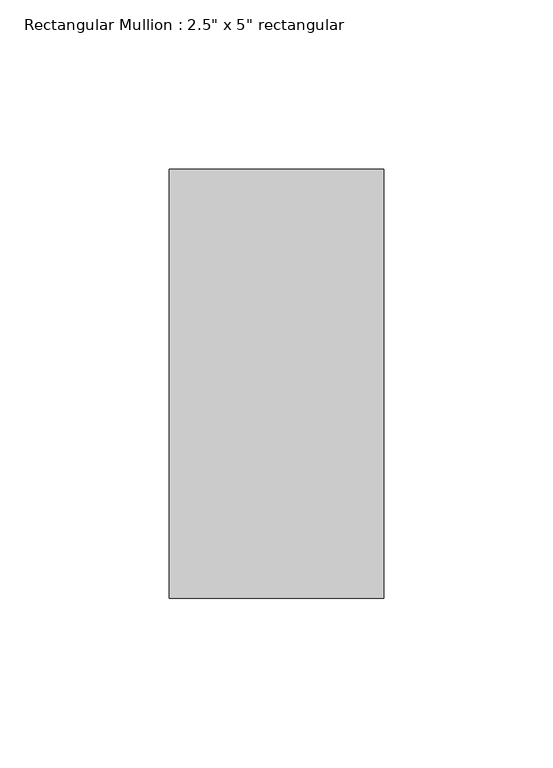
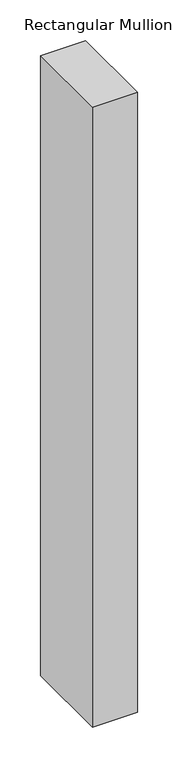
"""IFC4 building model written with IfcOpenShell, lengths in millimetres: member geometry."""

from ifc_helpers import new_model, si_unit, frame, origin, place, context, project, spatial, polyline, outline, extrude, source, transform, mapped, element, save


def member_f098b74a(model_context):
    return source(origin(), model_context, "Body", "SweptSolid", [
        extrude(outline(polyline([(31.75, 63.5), (31.75, -63.5), (-31.75, -63.5), (-31.75, 63.5), (31.75, 63.5)])), frame((0.0, 0.0, -927.3653615), z_axis=(0.0, 0.0, 1.0), x_axis=(1.0, 0.0, 0.0)), (0.0, 0.0, 1.0), 927.3653615),
    ])


if __name__ == "__main__":
    model = new_model("IFC4")
    model_context = context("Model", 3, world=origin())
    ifc_project = project(units=[si_unit("LENGTHUNIT", "METRE", prefix="MILLI")], contexts=[model_context])
    site = spatial("IfcSite", under=ifc_project)
    building = spatial("IfcBuilding", under=site)
    placement = place(None, origin())
    member_shape = member_f098b74a(model_context)
    element("IfcMember", 1, ObjectType="Rectangular Mullion : 2.5\" x 5\" rectangular", at=placement, inside=building, context=model_context, shape_type="MappedRepresentation", body=[
        mapped(member_shape, transform((0.0, 0.0, 0.0), x_axis=(1.0, 0.0, 0.0), y_axis=(0.0, 1.0, 0.0), z_axis=(0.0, 0.0, 1.0))),
    ])
    save(model, "model.ifc")

# Revit data of these elements
# Type "Rectangular Mullion : 2.5\" x 5\" rectangular"
#   built-in parameter 1007304 = 0.416667 (stored number, unit not read)
#   built-in parameter 1007301 = 0.104167 (stored number, unit not read)
#   built-in parameter 1007300 = 0.104167 (stored number, unit not read)
# Element 1 (IfcMember, "Rectangular Mullion : 2.5\" x 5\" rectangular")
#   Materials on its faces: "Aluminum"
# Materials
#   "Aluminum": class "Metal", colour RGB 247 247 247, transparency 0, Description = "Aluminum 6061", Cost = 0
